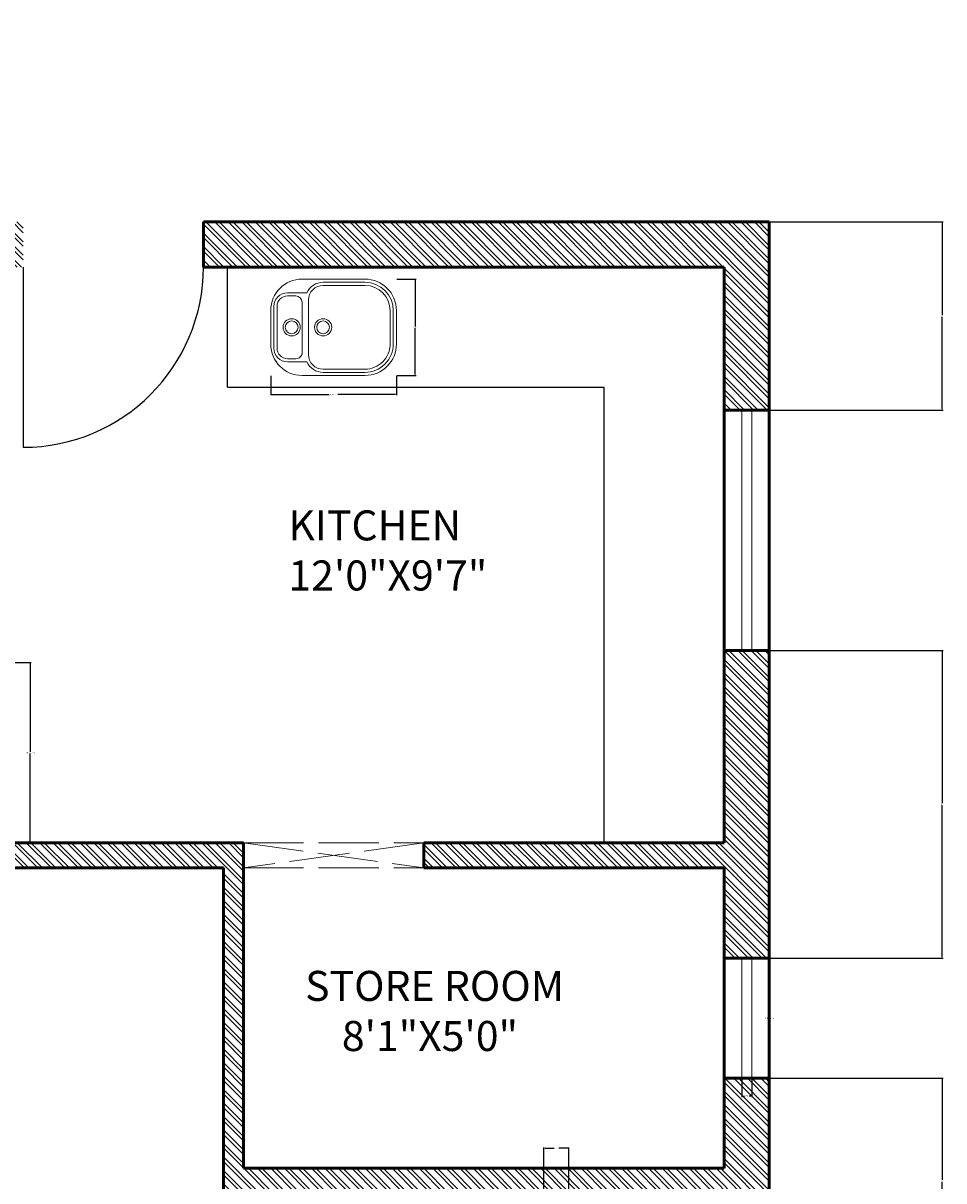
# Model space of a CAD drawing. Units: inches. Extents: x 10696 to 11614, y 5787 to 6498.
# Tile 5 of 9: x 10909 to 11093, y 6120 to 6351. Entities that reach past the tile are written whole.
import ezdxf

# ---------------------------------------------------------------- set-up
doc = ezdxf.new("R2010")
doc.units = ezdxf.units.IN
doc.linetypes.add('ACAD_ISO02W100', pattern=[15, 12, -3])
for name, color, linetype, lineweight in [('A-ANNO-DIMS', 2, 'Continuous', 18), ('A-AREA-IDEN', 7, 'Continuous', 25), ('A-DOOR', 3, 'Continuous', 25), ('A-FLOR-CASE', 32, 'Continuous', 25), ('A-FLOR-FIXT', 9, 'Continuous', 20), ('A-GLAZ', 4, 'Continuous', 20), ('A-WALL', 7, 'Continuous', 50), ('A-WALL-OVHD', 7, 'ACAD_ISO02W100', 18), ('A-WALL-PATT', 252, 'Continuous', 13)]:
    doc.layers.add(name, color=color, linetype=linetype, lineweight=lineweight)
doc.styles.get("Standard").update_dxf_attribs({"font": 'arial.ttf'})
doc.dimstyles.get("Standard").update_dxf_attribs({"dimtxt": 0.18, "dimasz": 0.18, "dimexe": 0.18, "dimexo": 0.0625, "dimgap": 0.09, "dimtad": 0, "dimtih": 1, "dimtoh": 1, "dimdec": 4, "dimzin": 0, "dimdsep": 46, "dimtxsty": 'Standard', "dimcen": 0.09, "dimadec": 0, "dimazin": 0, "dimtfac": 1, "dimtdec": 4, "dimtofl": 0, "dimtmove": 0, "dimatfit": 3, "dimfxl": 1, "dimtolj": 1, "dimtzin": 0, "dimarcsym": 0})

# ---------------------------------------------------------------- blocks, each defined once
blk = doc.blocks.new('A$C29210457')
for p, q in [((0.63, 0.644), (0.21, 0.644)), ((0.63, 0.623), (0.3499, 0.623)), ((0.2416, 0.553), (0.1119, 0.553)), ((0.63, 0.602), (0.35, 0.602)), ((0.168, 0.532), (0.112, 0.532)), ((0.14, 0.532), (0.14, 0.532)), ((0.21, 0.154), (0.21, 0.49)), ((0.252, 0.14), (0.252, 0.504)), ((0, 0.434), (0, 0.21)), ((0.021, 0.462), (0.021, 0.182)), ((0.042, 0.182), (0.042, 0.462)), ((0.798, 0.21), (0.798, 0.434)), ((0.819, 0.21), (0.819, 0.434)), ((0.84, 0.21), (0.84, 0.434)), ((0.2416, 0.091), (0.1119, 0.091)), ((0.168, 0.112), (0.112, 0.112)), ((0.14, 0.112), (0.14, 0.112)), ((0.63, 0), (0.21, 0)), ((0.63, 0.042), (0.35, 0.042)), ((0.63, 0.021), (0.35, 0.021))]:
    blk.add_line(p, q)
for centre, radius in [((0.14, 0.322), 0.0574), ((0.14, 0.322), 0.0427), ((0.35, 0.322), 0.0574), ((0.35, 0.322), 0.0427)]:
    blk.add_circle(centre, radius)
for centre, radius, start, end in [((0.21, 0.434), 0.21, 90, 180), ((0.35, 0.504), 0.119, 90.0649, 155.684), ((0.63, 0.434), 0.21, 0, 90), ((0.63, 0.434), 0.189, 0, 90), ((0.112, 0.462), 0.091, 90.0958, 180), ((0.35, 0.504), 0.098, 90, 180), ((0.63, 0.434), 0.168, 0, 90), ((0.112, 0.462), 0.07, 90, 180), ((0.168, 0.49), 0.042, 0.00002, 90), ((0.21, 0.21), 0.21, 180, 270), ((0.112, 0.182), 0.091, 180, 270), ((0.112, 0.182), 0.07, 180, 270), ((0.63, 0.21), 0.21, 270, 0.00001), ((0.63, 0.21), 0.168, 270, 0.00001), ((0.63, 0.21), 0.189, 270, 0.00001), ((0.168, 0.154), 0.042, 270, 0.00003), ((0.35, 0.14), 0.119, 204.316, 269.978), ((0.35, 0.14), 0.098, 180, 270)]:
    blk.add_arc(centre, radius, start, end)
blk = doc.blocks.new('A$C292E2DA8')
at = {"xscale": 729, "yscale": 729, "zscale": 729}
blk.add_blockref('A$C29210457', (0, 0), dxfattribs=at)
blk = doc.blocks.new('DOOR-SINGLE-36-KITCHEN')
blk.add_line((0, 36), (0, 0))
blk.add_arc((0, 36), 36, 270, 0)
blk = doc.blocks.new('WIN-GLAZ-24')
for p, q in [((0, 24), (0, 0)), ((2, 24), (2, 0))]:
    blk.add_line(p, q)
blk = doc.blocks.new('WIN-GLAZ-48')
for p, q in [((0, 48), (0, 0)), ((2, 48), (2, 0))]:
    blk.add_line(p, q)
blk = doc.blocks.new('KITCHEN-COUNTER-L')
for p, q in [((0, 91), (0, 115)), ((0, 91), (75.19, 91)), ((75.19, 0), (75.19, 91))]:
    blk.add_line(p, q)
blk = doc.blocks.new('OPENING-OVHD-36X5')
for p, q in [((0, 5), (36, 5)), ((36, 5), (0, 0)), ((0, 5), (36, 0)), ((0, 0), (36, 0))]:
    blk.add_line(p, q)
blk = doc.blocks.new('*D30')
at = {"layer": 'A-ANNO-DIMS', "color": 0, "lineweight": -2, "transparency": 16777216}
for p, q in [((11054.48, 6164.07), (11058.19, 6164.07)), ((11058.01, 6163.89), (11058.01, 6152.25)), ((11058.01, 6140.25), (11058.01, 6151.89)), ((11054.48, 6140.07), (11058.19, 6140.07))]:
    blk.add_line(p, q, dxfattribs=at)
at = {"layer": 'A-ANNO-DIMS', "color": 0, "transparency": 16777216}
for points in [[(11057.98, 6163.89), (11058.04, 6163.89), (11058.01, 6164.07)], [(11057.98, 6140.25), (11058.04, 6140.25), (11058.01, 6140.07)]]:
    blk.add_solid(points, dxfattribs=at)
at = {"layer": 'Defpoints', "color": 0, "transparency": 16777216}
for p in [(11054.41, 6164.07), (11058.01, 6164.07), (11054.41, 6140.07)]:
    blk.add_point(p, dxfattribs=at)
at = {"layer": 'A-ANNO-DIMS', "color": 0, "transparency": 16777216, "insert": (11058.01, 6152.07), "char_height": 0.18, "attachment_point": 5}
blk.add_mtext('\\A1;WINDOW 24 TYP.', dxfattribs=at)
blk = doc.blocks.new('*D31')
at = {"layer": 'A-ANNO-DIMS', "color": 0, "lineweight": -2, "transparency": 16777216}
for p, q in [((11052.41, 6140.01), (11052.41, 6136.29)), ((11054.41, 6140.01), (11054.41, 6136.29)), ((11052.59, 6136.47), (11052.95, 6136.47)), ((11054.23, 6136.47), (11053.87, 6136.47))]:
    blk.add_line(p, q, dxfattribs=at)
at = {"layer": 'A-ANNO-DIMS', "color": 0, "transparency": 16777216}
for points in [[(11052.59, 6136.5), (11052.59, 6136.44), (11052.41, 6136.47)], [(11054.23, 6136.5), (11054.23, 6136.44), (11054.41, 6136.47)]]:
    blk.add_solid(points, dxfattribs=at)
at = {"layer": 'Defpoints', "color": 0, "transparency": 16777216}
for p in [(11052.41, 6140.07), (11054.41, 6140.07), (11054.41, 6136.47)]:
    blk.add_point(p, dxfattribs=at)
at = {"layer": 'A-ANNO-DIMS', "color": 0, "transparency": 16777216, "insert": (11053.41, 6136.47), "char_height": 0.18, "attachment_point": 5}
blk.add_mtext('\\A1;2 TYP.', dxfattribs=at)
blk = doc.blocks.new('*D40')
at = {"layer": 'A-ANNO-DIMS', "color": 0, "lineweight": -2, "transparency": 16777216}
for p, q in [((10958.35, 6280.35), (10958.35, 6276.47)), ((10983.45, 6280.35), (10983.45, 6276.47)), ((10958.53, 6276.65), (10970.05, 6276.65)), ((10983.27, 6276.65), (10971.76, 6276.65))]:
    blk.add_line(p, q, dxfattribs=at)
at = {"layer": 'A-ANNO-DIMS', "color": 0, "transparency": 16777216}
for points in [[(10958.53, 6276.68), (10958.53, 6276.62), (10958.35, 6276.65)], [(10983.27, 6276.68), (10983.27, 6276.62), (10983.45, 6276.65)]]:
    blk.add_solid(points, dxfattribs=at)
at = {"layer": 'Defpoints', "color": 0, "transparency": 16777216}
for p in [(10958.35, 6280.42), (10983.45, 6280.42), (10983.45, 6276.65)]:
    blk.add_point(p, dxfattribs=at)
at = {"layer": 'A-ANNO-DIMS', "color": 0, "transparency": 16777216, "insert": (10970.9, 6276.65), "char_height": 0.18, "attachment_point": 5}
blk.add_mtext('\\A1;SINK 25 TYP.', dxfattribs=at)
blk = doc.blocks.new('*D41')
at = {"layer": 'A-ANNO-DIMS', "color": 0, "lineweight": -2, "transparency": 16777216}
for p, q in [((10983.51, 6299.66), (10987.39, 6299.66)), ((10987.21, 6299.48), (10987.21, 6290.22)), ((10987.21, 6280.6), (10987.21, 6289.86)), ((10983.51, 6280.42), (10987.39, 6280.42))]:
    blk.add_line(p, q, dxfattribs=at)
at = {"layer": 'A-ANNO-DIMS', "color": 0, "transparency": 16777216}
for points in [[(10987.18, 6299.48), (10987.24, 6299.48), (10987.21, 6299.66)], [(10987.18, 6280.6), (10987.24, 6280.6), (10987.21, 6280.42)]]:
    blk.add_solid(points, dxfattribs=at)
at = {"layer": 'Defpoints', "color": 0, "transparency": 16777216}
for p in [(10983.45, 6299.66), (10987.21, 6299.66), (10983.45, 6280.42)]:
    blk.add_point(p, dxfattribs=at)
at = {"layer": 'A-ANNO-DIMS', "color": 0, "transparency": 16777216, "insert": (10987.21, 6290.04), "char_height": 0.18, "attachment_point": 5}
blk.add_mtext('\\A1;19 TYP.', dxfattribs=at)
blk = doc.blocks.new('*D61')
at = {"layer": 'A-ANNO-DIMS', "color": 0, "lineweight": -2, "transparency": 16777216}
for p, q in [((11012.91, 6117.13), (11012.91, 6126.25)), ((11013.09, 6126.07), (11014.95, 6126.07)), ((11017.73, 6126.07), (11015.87, 6126.07)), ((11017.91, 6117.13), (11017.91, 6126.25))]:
    blk.add_line(p, q, dxfattribs=at)
at = {"layer": 'A-ANNO-DIMS', "color": 0, "transparency": 16777216}
for points in [[(11013.09, 6126.1), (11013.09, 6126.04), (11012.91, 6126.07)], [(11017.73, 6126.1), (11017.73, 6126.04), (11017.91, 6126.07)]]:
    blk.add_solid(points, dxfattribs=at)
at = {"layer": 'Defpoints', "color": 0, "transparency": 16777216}
for p in [(11017.91, 6126.07), (11012.91, 6117.07), (11017.91, 6117.07)]:
    blk.add_point(p, dxfattribs=at)
at = {"layer": 'A-ANNO-DIMS', "color": 0, "transparency": 16777216, "insert": (11015.41, 6126.07), "char_height": 0.18, "attachment_point": 5}
blk.add_mtext('\\A1;5 TYP.', dxfattribs=at)
blk = doc.blocks.new('*D64')
at = {"layer": 'A-ANNO-DIMS', "color": 0, "lineweight": -2, "transparency": 16777216}
for p, q in [((10904.98, 6223.07), (10910.49, 6223.07)), ((10910.31, 6222.89), (10910.31, 6205.25)), ((10910.31, 6187.25), (10910.31, 6204.89)), ((10904.98, 6187.07), (10910.49, 6187.07))]:
    blk.add_line(p, q, dxfattribs=at)
at = {"layer": 'A-ANNO-DIMS', "color": 0, "transparency": 16777216}
for points in [[(10910.28, 6222.89), (10910.34, 6222.89), (10910.31, 6223.07)], [(10910.28, 6187.25), (10910.34, 6187.25), (10910.31, 6187.07)]]:
    blk.add_solid(points, dxfattribs=at)
at = {"layer": 'Defpoints', "color": 0, "transparency": 16777216}
for p in [(10904.91, 6223.07), (10910.31, 6223.07), (10904.91, 6187.07)]:
    blk.add_point(p, dxfattribs=at)
at = {"layer": 'A-ANNO-DIMS', "color": 0, "transparency": 16777216, "insert": (10910.31, 6205.07), "char_height": 0.18, "attachment_point": 5}
blk.add_mtext('\\A1;OPENING 36 TYP.', dxfattribs=at)
blk = doc.blocks.new('*D89')
at = {"layer": 'A-ANNO-DIMS', "color": 0, "lineweight": -2, "transparency": 16777216}
for p, q in [((11057.98, 6140.07), (11092.64, 6140.07)), ((11092.46, 6139.89), (11092.46, 6119.75)), ((11092.46, 6099.25), (11092.46, 6119.39)), ((11057.98, 6099.07), (11092.64, 6099.07))]:
    blk.add_line(p, q, dxfattribs=at)
at = {"layer": 'A-ANNO-DIMS', "color": 0, "transparency": 16777216}
for points in [[(11092.43, 6139.89), (11092.49, 6139.89), (11092.46, 6140.07)], [(11092.43, 6099.25), (11092.49, 6099.25), (11092.46, 6099.07)]]:
    blk.add_solid(points, dxfattribs=at)
at = {"layer": 'Defpoints', "color": 0, "transparency": 16777216}
for p in [(11057.91, 6140.07), (11092.46, 6140.07), (11057.91, 6099.07)]:
    blk.add_point(p, dxfattribs=at)
at = {"layer": 'A-ANNO-DIMS', "color": 0, "transparency": 16777216, "insert": (11092.46, 6119.57), "char_height": 0.18, "attachment_point": 5}
blk.add_mtext('\\A1;41', dxfattribs=at)
blk = doc.blocks.new('*D90')
at = {"layer": 'A-ANNO-DIMS', "color": 0, "lineweight": -2, "transparency": 16777216}
for p, q in [((11057.98, 6225.51), (11092.64, 6225.51)), ((11092.46, 6225.33), (11092.46, 6194.97)), ((11092.46, 6164.25), (11092.46, 6194.61)), ((11057.98, 6164.07), (11092.64, 6164.07))]:
    blk.add_line(p, q, dxfattribs=at)
at = {"layer": 'A-ANNO-DIMS', "color": 0, "transparency": 16777216}
for points in [[(11092.43, 6225.33), (11092.49, 6225.33), (11092.46, 6225.51)], [(11092.43, 6164.25), (11092.49, 6164.25), (11092.46, 6164.07)]]:
    blk.add_solid(points, dxfattribs=at)
at = {"layer": 'Defpoints', "color": 0, "transparency": 16777216}
for p in [(11057.91, 6225.51), (11092.46, 6225.51), (11057.91, 6164.07)]:
    blk.add_point(p, dxfattribs=at)
at = {"layer": 'A-ANNO-DIMS', "color": 0, "transparency": 16777216, "insert": (11092.46, 6194.79), "char_height": 0.18, "attachment_point": 5}
blk.add_mtext('\\A1;61.44', dxfattribs=at)
blk = doc.blocks.new('*D91')
at = {"layer": 'A-ANNO-DIMS', "color": 0, "lineweight": -2, "transparency": 16777216}
for p, q in [((11057.98, 6311.07), (11092.64, 6311.07)), ((11092.46, 6310.89), (11092.46, 6292.47)), ((11092.46, 6273.69), (11092.46, 6292.11)), ((11057.98, 6273.51), (11092.64, 6273.51))]:
    blk.add_line(p, q, dxfattribs=at)
at = {"layer": 'A-ANNO-DIMS', "color": 0, "transparency": 16777216}
for points in [[(11092.43, 6310.89), (11092.49, 6310.89), (11092.46, 6311.07)], [(11092.43, 6273.69), (11092.49, 6273.69), (11092.46, 6273.51)]]:
    blk.add_solid(points, dxfattribs=at)
at = {"layer": 'Defpoints', "color": 0, "transparency": 16777216}
for p in [(11057.91, 6311.07), (11092.46, 6311.07), (11057.91, 6273.51)]:
    blk.add_point(p, dxfattribs=at)
at = {"layer": 'A-ANNO-DIMS', "color": 0, "transparency": 16777216, "insert": (11092.46, 6292.29), "char_height": 0.18, "attachment_point": 5}
blk.add_mtext('\\A1;37.56', dxfattribs=at)

msp = doc.modelspace()

# ---------------------------------------------------------------- hatches: boundary and pattern name
at = {"layer": 'A-WALL-PATT'}
h = msp.add_hatch(dxfattribs=at)
h.set_pattern_fill('ANSI32', color=256, scale=0.2, angle=90)
h.paths.add_polyline_path([(10767.913, 5961.07), (10739.913, 5961.07), (10739.913, 6001.333), (10730.913, 6001.333), (10730.913, 5887.07), (10739.913, 5887.07), (10739.913, 5952.07), (10767.913, 5952.07)])
h.paths.add_polyline_path([(10739.913, 6127.055), (10730.913, 6127.055), (10730.913, 6073.333), (10739.913, 6073.333)])
h.paths.add_polyline_path([(10739.913, 6267.869, -0.035413), (10740.694, 6278.876), (10731.784, 6280.146, 0.035413), (10730.913, 6267.869), (10730.913, 6199.055), (10739.913, 6199.055)])
h.paths.add_polyline_path([(10794.29, 6342.205), (10791.564, 6350.783, 0.1142038), (10757.817, 6330.777), (10764.034, 6324.269, -0.1142038)])
h.paths.add_polyline_path([(10844.262, 6350.783), (10841.536, 6342.205, -0.065871), (10860.057, 6333.503), (10864.919, 6341.077, 0.065871)])
h.paths.add_polyline_path([(10908.913, 6311.07), (10895.913, 6311.07), (10895.913, 6306.404, 0.0519949), (10886.285, 6321.667), (10879.212, 6316.101, -0.1682272), (10895.913, 6267.869), (10895.913, 6223.07), (10904.913, 6223.07), (10904.913, 6302.07), (10908.913, 6302.07)])
h.paths.add_polyline_path([(11057.913, 6311.07), (10944.913, 6311.07), (10944.913, 6302.07), (11048.913, 6302.07), (11048.913, 6273.514), (11057.913, 6273.514)])
h.paths.add_polyline_path([(11057.913, 6225.514), (11048.913, 6225.514), (11048.913, 6187.07), (10988.913, 6187.07), (10988.913, 6182.07), (11048.913, 6182.07), (11048.913, 6164.07), (11057.913, 6164.07)])
h.paths.add_polyline_path([(10952.913, 6187.07), (10895.913, 6187.07), (10895.913, 6182.07), (10948.913, 6182.07), (10948.913, 6113.07), (10952.913, 6113.07), (10952.913, 6117.07), (11048.913, 6117.07), (11048.913, 6099.07), (11057.913, 6099.07), (11057.913, 6140.07), (11048.913, 6140.07), (11048.913, 6122.07), (10952.913, 6122.07)])
h.paths.add_polyline_path([(11057.913, 6075.07), (11048.913, 6075.07), (11048.913, 6057.07), (10952.913, 6057.07), (10952.913, 6083.07), (10944.913, 6083.07), (10944.913, 6078.07), (10948.913, 6078.07), (10948.913, 6052.07), (11048.913, 6052.07), (11048.913, 6028.07), (11057.913, 6028.07)])
h.paths.add_polyline_path([(11057.913, 5992.07), (11048.913, 5992.07), (11048.913, 5896.07), (11000.913, 5896.07), (11000.913, 5887.07), (11057.913, 5887.07)])
h.paths.add_polyline_path([(10952.913, 5896.07), (10904.913, 5896.07), (10904.913, 6078.07), (10908.913, 6078.07), (10908.913, 6083.07), (10899.913, 6083.07), (10899.913, 5961.07), (10891.913, 5961.07), (10891.913, 5952.07), (10895.913, 5952.07), (10895.913, 5887.07), (10952.913, 5887.07)])
h.paths.add_polyline_path([(10843.913, 5961.07), (10815.913, 5961.07), (10815.913, 5952.07), (10843.913, 5952.07)])

# ---------------------------------------------------------------- linework, layer by layer
at = {"layer": 'A-WALL'}
for p, q in [((10944.913, 6302.07), (10944.913, 6311.07)), ((10944.913, 6311.07), (11057.913, 6311.07)), ((11057.913, 5887.07), (11057.913, 6311.07)), ((10944.913, 6302.07), (11048.913, 6302.07)), ((11048.913, 6187.07), (11048.913, 6302.07)), ((11048.913, 6273.514), (11057.913, 6273.514)), ((11048.913, 6225.514), (11057.913, 6225.514)), ((10895.913, 6187.07), (10952.913, 6187.07)), ((10952.913, 6122.07), (10952.913, 6187.07)), ((10988.913, 6182.07), (10988.913, 6187.07)), ((10988.913, 6187.07), (11048.913, 6187.07)), ((10895.913, 6182.07), (10948.913, 6182.07)), ((10948.913, 6113.07), (10948.913, 6182.07)), ((10988.913, 6182.07), (11048.913, 6182.07)), ((11048.913, 6122.07), (11048.913, 6182.07)), ((11048.913, 6164.07), (11057.913, 6164.07)), ((11048.913, 6140.07), (11057.913, 6140.07)), ((10952.913, 6122.07), (11048.913, 6122.07))]:
    msp.add_line(p, q, dxfattribs=at)

# ---------------------------------------------------------------- block references
at = {"layer": 'A-DOOR'}
msp.add_blockref('DOOR-SINGLE-36-KITCHEN', (10908.913, 6266.07), dxfattribs=at)
at = {"layer": 'A-FLOR-CASE'}
msp.add_blockref('KITCHEN-COUNTER-L', (10949.723, 6187.07), dxfattribs=at)
at = {"layer": 'A-FLOR-FIXT', "xscale": 0.0409818961513061, "yscale": 0.0409818961513061, "zscale": 0.0409818961513061}
msp.add_blockref('A$C292E2DA8', (10958.354, 6280.417), dxfattribs=at)
at = {"layer": 'A-GLAZ'}
for name, p in [('WIN-GLAZ-48', (11052.413, 6225.514)), ('WIN-GLAZ-24', (11052.413, 6140.07))]:
    msp.add_blockref(name, p, dxfattribs=at)
at = {"layer": 'A-WALL-OVHD'}
msp.add_blockref('OPENING-OVHD-36X5', (10952.913, 6182.07), dxfattribs=at)

# ---------------------------------------------------------------- texts
at = {"layer": 'A-AREA-IDEN', "char_height": 6, "attachment_point": 1}
for s, width, insert in [('KITCHEN\\P12\'0"X9\'7"', 38.38274, (10961.883, 6253.474)), ('STORE ROOM\\P    8\'1"X5\'0"', 59.23595, (10965.221, 6161.5))]:
    msp.add_mtext_dynamic_manual_height_columns(s, width=width, gutter_width=12.5, heights=[0], dxfattribs=dict(at, insert=insert))

# ---------------------------------------------------------------- dimensions: what is measured, and where the dimension line sits
at = {"layer": 'A-ANNO-DIMS'}
for base, p1, p2, override, picture, middle in [((11092.463, 6311.07), (11057.913, 6273.514), (11057.913, 6311.07), {"dimdec": 2, "dimlfac": 1, "dimrnd": 0, "dimzin": 0, "dimdsep": 46, "dimlunit": 2}, '*D91', (11092.463, 6292.292)), ((11092.463, 6225.514), (11057.913, 6164.07), (11057.913, 6225.514), {"dimdec": 2, "dimlfac": 1, "dimrnd": 0, "dimzin": 0, "dimdsep": 46, "dimlunit": 2}, '*D90', (11092.463, 6194.792)), ((11092.463, 6140.07), (11057.913, 6099.07), (11057.913, 6140.07), {"dimdec": 0, "dimlfac": 1, "dimrnd": 0, "dimzin": 0, "dimdsep": 46, "dimlunit": 2}, '*D89', (11092.463, 6119.57))]:
    dim = msp.add_linear_dim(base=base, p1=p1, p2=p2, angle=90, dimstyle='Standard', override=override, dxfattribs=at)
    dim.commit()
    dim.dimension.update_dxf_attribs({"geometry": picture, "text_midpoint": middle})
for base, p1, p2, text, picture, middle in [((10987.214, 6299.657), (10983.449, 6280.417), (10983.449, 6299.657), '<> TYP.', '*D41', (10987.214, 6290.037)), ((10910.313, 6223.07), (10904.913, 6187.07), (10904.913, 6223.07), 'OPENING <> TYP.', '*D64', (10910.313, 6205.07)), ((11058.013, 6164.07), (11054.413, 6140.07), (11054.413, 6164.07), 'WINDOW <> TYP.', '*D30', (11058.013, 6152.07))]:
    dim = msp.add_linear_dim(base=base, p1=p1, p2=p2, angle=90, text=text, dimstyle='Standard', override={"dimdec": 0, "dimlfac": 1, "dimrnd": 0, "dimzin": 0, "dimdsep": 46, "dimlunit": 2}, dxfattribs=at)
    dim.commit()
    dim.dimension.update_dxf_attribs({"geometry": picture, "text_midpoint": middle})
for base, p1, p2, text, picture, middle in [((10983.449, 6276.652), (10958.354, 6280.417), (10983.449, 6280.417), 'SINK <> TYP.', '*D40', (10970.901, 6276.652)), ((11054.413, 6136.47), (11052.413, 6140.07), (11054.413, 6140.07), '<> TYP.', '*D31', (11053.413, 6136.47)), ((11017.913, 6126.07), (11012.913, 6117.07), (11017.913, 6117.07), '<> TYP.', '*D61', (11015.413, 6126.07))]:
    dim = msp.add_linear_dim(base=base, p1=p1, p2=p2, text=text, dimstyle='Standard', override={"dimdec": 0, "dimlfac": 1, "dimrnd": 0, "dimzin": 0, "dimdsep": 46, "dimlunit": 2}, dxfattribs=at)
    dim.commit()
    dim.dimension.update_dxf_attribs({"geometry": picture, "text_midpoint": middle})

doc.saveas('drawing.dxf')
